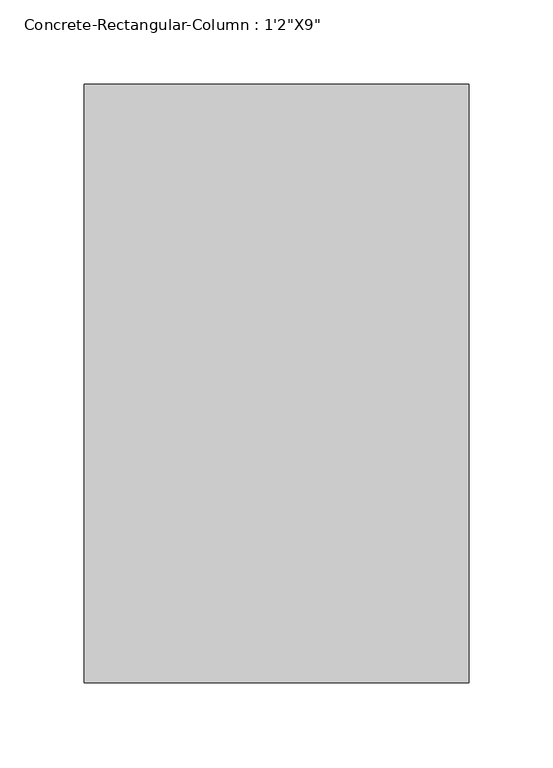
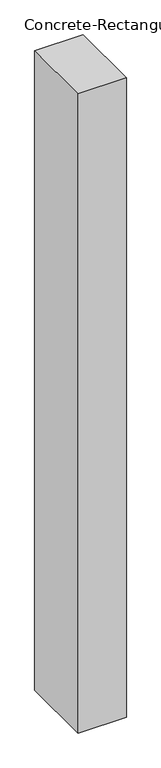
"""IFC4 building model written with IfcOpenShell, lengths in millimetres: column geometry."""

from ifc_helpers import new_model, si_unit, frame, origin, place, context, project, spatial, polyline, outline, extrude, source, transform, mapped, element, save


def column_4105a6de(model_context):
    return source(origin(), model_context, "Body", "SweptSolid", [
        extrude(outline(polyline([(114.3, 177.8), (114.3, -177.8), (-114.3, -177.8), (-114.3, 177.8), (114.3, 177.8)])), frame((0.0, 0.0, 6400.8), z_axis=(0.0, 0.0, 1.0), x_axis=(1.0, 0.0, 0.0)), (0.0, 0.0, 1.0), 3200.4),
    ])


if __name__ == "__main__":
    model = new_model("IFC4")
    model_context = context("Model", 3, world=origin())
    ifc_project = project(units=[si_unit("LENGTHUNIT", "METRE", prefix="MILLI")], contexts=[model_context])
    site = spatial("IfcSite", under=ifc_project)
    building = spatial("IfcBuilding", under=site)
    placement = place(None, origin())
    column_shape = column_4105a6de(model_context)
    element("IfcColumn", 1, ObjectType="Concrete-Rectangular-Column : 1'2\"X9\"", at=placement, inside=building, context=model_context, shape_type="MappedRepresentation", body=[
        mapped(column_shape, transform((0.0, 0.0, 0.0), x_axis=(1.0, 0.0, 0.0), y_axis=(0.0, 1.0, 0.0), z_axis=(0.0, 0.0, 1.0))),
    ])
    save(model, "model.ifc")

# Revit data of these elements
# Type "Concrete-Rectangular-Column : 1'2\"X9\""
#   Assembly Code = "B10"
#   b = 0' - 9"
#   h = 1' - 2"
#   Structural Material [instance default] = Concrete, Cast-in-Place gray
# Element 1 (IfcColumn, "Concrete-Rectangular-Column : 1'2\"X9\"")
#   Materials on its faces: "Concrete, Cast-in-Place gray"
# Materials
#   "Concrete, Cast-in-Place gray": class "Concrete", colour RGB 192 192 192, transparency 0, Description = "Cast-in-place concrete", Cost = 0
